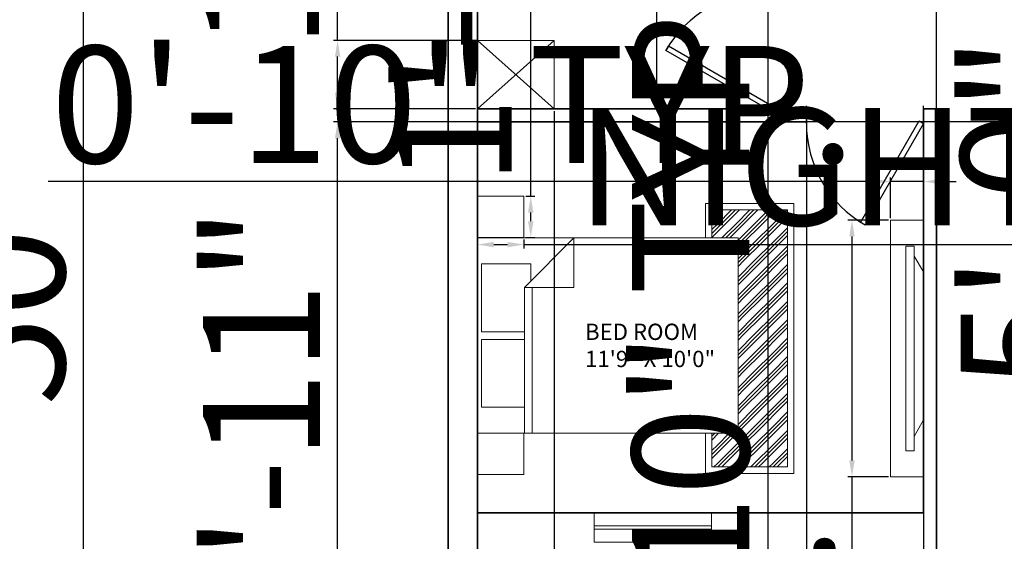
# Model space of a CAD drawing. Units: inches. Extents: x 2901 to 21549, y 2042 to 3828.
# Tile 3 of 10: x 3202 to 3505, y 3099 to 3259. Entities that reach past the tile are written whole.
import ezdxf

# ---------------------------------------------------------------- set-up
doc = ezdxf.new("R2010")
doc.units = ezdxf.units.IN
doc.layers.get('Defpoints').update_dxf_attribs({"color": 1})
for name, color, linetype, lineweight in [('A-ANNO-DIMS', 2, 'Continuous', 18), ('A-AREA-IDEN', 7, 'Continuous', 18), ('A-DOOR', 3, 'Continuous', 25), ('A-EQPM', 8, 'Continuous', 18), ('A-FLOR-FIXT', 9, 'Continuous', 18), ('A-FLOR-PATT', 252, 'Continuous', 13), ('A-FURN', 8, 'Continuous', 18), ('A-GLAZ', 4, 'Continuous', 18), ('A-WALL', 7, 'Continuous', 35)]:
    doc.layers.add(name, color=color, linetype=linetype, lineweight=lineweight)
doc.styles.get("Standard").update_dxf_attribs({"font": 'arial.ttf'})
doc.dimstyles.new('ISO-25', dxfattribs={"dimtxt": 36, "dimasz": 5, "dimexe": 1.25, "dimexo": 0.625, "dimtad": 1, "dimdec": 0, "dimlunit": 3, "dimtxsty": 'Standard', "dimcen": 2.5, "dimadec": 0, "dimazin": 0, "dimtfac": 1, "dimtdec": 0, "dimtmove": 0, "dimatfit": 3, "dimfxl": 1, "dimarcsym": 0})

# ---------------------------------------------------------------- blocks, each defined once
blk = doc.blocks.new('*U22')
for p, q in [((-40, 0), (-40, 6)), ((0, 0), (0, 6))]:
    blk.add_line(p, q)
blk.add_lwpolyline([(0, 0), (-20, -34.64), (-21.52, -33.77), (-1.52, 0.87)], close=True)
blk.add_arc((0, 0), 40, 180, 240)
blk = doc.blocks.new('Bed - Queen')
for p, q in [((0, -80.00003), (0, 0)), ((0, 0), (59.99999, 0)), ((59.99999, 0), (59.99999, -80.00003)), ((7.99999, -1.2), (28.79998, -1.2)), ((7.99999, -14.4), (7.99999, -1.2)), ((28.79998, -1.2), (28.79998, -14.4)), ((31.19999, -1.2), (51.99999, -1.2)), ((31.19999, -14.4), (31.19999, -1.2)), ((51.99999, -1.2), (51.99999, -16.4)), ((0, -14.4), (44.8, -14.4)), ((59.99999, -29.6), (44.8, -14.4)), ((44.8, -14.4), (44.8, -29.6)), ((44.8, -16.8), (0, -16.8)), ((51.99999, -16.4), (46.79936, -16.4)), ((44.8, -29.6), (59.99999, -29.6)), ((59.99999, -80.00003), (0, -80.00003))]:
    blk.add_line(p, q)
blk = doc.blocks.new('*D31')
at = {"layer": 'A-ANNO-DIMS', "color": 0, "lineweight": -2, "transparency": 16777216}
for p, q in [((3333.44, 3474.48), (3220.78, 3474.48)), ((3222.03, 3469.48), (3222.03, 2879.48)), ((3333.44, 2874.48), (3220.78, 2874.48))]:
    blk.add_line(p, q, dxfattribs=at)
at = {"layer": 'A-ANNO-DIMS', "color": 0, "transparency": 16777216}
for points in [[(3221.19, 3469.48), (3222.86, 3469.48), (3222.03, 3474.48)], [(3221.19, 2879.48), (3222.86, 2879.48), (3222.03, 2874.48)]]:
    blk.add_solid(points, dxfattribs=at)
at = {"layer": 'Defpoints', "color": 0, "transparency": 16777216}
for p in [(3334.07, 3474.48), (3222.03, 2874.48), (3334.07, 2874.48)]:
    blk.add_point(p, dxfattribs=at)
at = {"layer": 'A-ANNO-DIMS', "color": 0, "transparency": 16777216, "insert": (3203.02, 3174.48), "char_height": 36, "attachment_point": 5, "rotation": 90}
blk.add_mtext("50'", dxfattribs=at)
blk = doc.blocks.new('WIN-36IN-9IN-WALL')
for p, q in [((0, 36), (9, 36)), ((0, 0), (0, 36)), ((4, 0), (4, 36)), ((5, 36), (5, 0)), ((9, 36), (9, 0)), ((9, 0), (0, 0))]:
    blk.add_line(p, q)
blk = doc.blocks.new('TABLE-BEDSIDE')
blk.add_lwpolyline([(0, 12.7), (14.22, 12.7), (14.22, 0), (0, 0)], close=True)
blk = doc.blocks.new('BEDROOM-MEDIA-UNIT')
for p, q in [((2.89, 66.49), (0, 61.37)), ((0, 15.88), (2.89, 11.11))]:
    blk.add_line(p, q)
for points in [[(0.06, 78.84), (10.18, 78.84), (10.18, 0), (0.06, 0)], [(2.89, 70.84), (5.46, 70.84), (5.46, 8), (2.89, 8)]]:
    blk.add_lwpolyline(points, close=True)
blk = doc.blocks.new('*D38')
at = {"layer": 'A-ANNO-DIMS', "color": 0, "lineweight": -2, "transparency": 16777216}
for p, q in [((3343.07, 3191.34), (3343.07, 3188.58)), ((3348.07, 3189.83), (3352.29, 3189.83)), ((3357.29, 3191.34), (3357.29, 3188.58)), ((3357.29, 3189.83), (3922.11, 3189.83))]:
    blk.add_line(p, q, dxfattribs=at)
at = {"layer": 'A-ANNO-DIMS', "color": 0, "transparency": 16777216}
for points in [[(3348.07, 3190.67), (3348.07, 3189), (3343.07, 3189.83)], [(3352.29, 3190.67), (3352.29, 3189), (3357.29, 3189.83)]]:
    blk.add_solid(points, dxfattribs=at)
at = {"layer": 'Defpoints', "color": 0, "transparency": 16777216}
for p in [(3343.07, 3191.97), (3357.29, 3191.97), (3357.29, 3189.83)]:
    blk.add_point(p, dxfattribs=at)
at = {"layer": 'A-ANNO-DIMS', "color": 0, "transparency": 16777216, "insert": (3642.2, 3209.07), "char_height": 36, "attachment_point": 5}
blk.add_mtext('NIGHTSTAND 1\'-2" TYP.', dxfattribs=at)
blk = doc.blocks.new('*D39')
at = {"layer": 'A-ANNO-DIMS', "color": 0, "lineweight": -2, "transparency": 16777216}
for p, q in [((3359.43, 3204.67), (3359.43, 3510.85)), ((3357.92, 3204.67), (3360.68, 3204.67)), ((3359.43, 3196.97), (3359.43, 3199.67)), ((3357.92, 3191.97), (3360.68, 3191.97))]:
    blk.add_line(p, q, dxfattribs=at)
at = {"layer": 'A-ANNO-DIMS', "color": 0, "transparency": 16777216}
for points in [[(3358.59, 3199.67), (3360.26, 3199.67), (3359.43, 3204.67)], [(3358.59, 3196.97), (3360.26, 3196.97), (3359.43, 3191.97)]]:
    blk.add_solid(points, dxfattribs=at)
at = {"layer": 'Defpoints', "color": 0, "transparency": 16777216}
for p in [(3357.29, 3204.67), (3359.43, 3204.67), (3357.29, 3191.97)]:
    blk.add_point(p, dxfattribs=at)
at = {"layer": 'A-ANNO-DIMS', "color": 0, "transparency": 16777216, "insert": (3340.19, 3360.26), "char_height": 36, "attachment_point": 5, "rotation": 90}
blk.add_mtext('1\'-0 1/2" TYP.', dxfattribs=at)
blk = doc.blocks.new('*D40')
at = {"layer": 'A-ANNO-DIMS', "color": 0, "lineweight": -2, "transparency": 16777216}
for p, q in [((3343.07, 3272.69), (3343.07, 3267.11)), ((3376.12, 3272.69), (3376.12, 3267.11)), ((3343.07, 3268.36), (3018.15, 3268.36)), ((3371.12, 3268.36), (3348.07, 3268.36))]:
    blk.add_line(p, q, dxfattribs=at)
at = {"layer": 'A-ANNO-DIMS', "color": 0, "transparency": 16777216}
for points in [[(3348.07, 3269.19), (3348.07, 3267.52), (3343.07, 3268.36)], [(3371.12, 3269.19), (3371.12, 3267.52), (3376.12, 3268.36)]]:
    blk.add_solid(points, dxfattribs=at)
at = {"layer": 'Defpoints', "color": 0, "transparency": 16777216}
for p in [(3343.07, 3273.32), (3376.12, 3273.32), (3343.07, 3268.36)]:
    blk.add_point(p, dxfattribs=at)
at = {"layer": 'A-ANNO-DIMS', "color": 0, "transparency": 16777216, "insert": (3178.11, 3287.6), "char_height": 36, "attachment_point": 5}
blk.add_mtext('WC 2\'-9" TYP.', dxfattribs=at)
blk = doc.blocks.new('*D42')
at = {"layer": 'A-ANNO-DIMS', "color": 0, "lineweight": -2, "transparency": 16777216}
for p, q in [((3533.42, 3266.44), (3528.38, 3599.53)), ((3535.49, 3266.47), (3532.17, 3266.42)), ((3533.62, 3253.49), (3533.5, 3261.44)), ((3535.76, 3248.52), (3532.44, 3248.47))]:
    blk.add_line(p, q, dxfattribs=at)
at = {"layer": 'A-ANNO-DIMS', "color": 0, "transparency": 16777216}
for points in [[(3534.33, 3261.45), (3532.66, 3261.43), (3533.42, 3266.44)], [(3534.45, 3253.5), (3532.78, 3253.48), (3533.69, 3248.49)]]:
    blk.add_solid(points, dxfattribs=at)
at = {"layer": 'Defpoints', "color": 0, "transparency": 16777216}
for p in [(3533.42, 3266.44), (3536.11, 3266.48), (3536.39, 3248.53)]:
    blk.add_point(p, dxfattribs=at)
at = {"layer": 'A-ANNO-DIMS', "color": 0, "transparency": 16777216, "insert": (3549.86, 3435.77), "char_height": 36, "attachment_point": 5, "rotation": 270.8679}
blk.add_mtext('LAV 1\'-6" TYP.', dxfattribs=at)
blk = doc.blocks.new('*D44')
at = {"layer": 'A-ANNO-DIMS', "color": 0, "lineweight": -2, "transparency": 16777216}
for p, q in [((3432.19, 3305.97), (3432.19, 3310.97)), ((3431.32, 3300.97), (3433.44, 3300.97)), ((3432.19, 3300.97), (3432.19, 3290.97)), ((3431.32, 3290.97), (3433.44, 3290.97)), ((3432.19, 3285.97), (3432.19, 2919.63))]:
    blk.add_line(p, q, dxfattribs=at)
at = {"layer": 'A-ANNO-DIMS', "color": 0, "transparency": 16777216}
for points in [[(3431.36, 3305.97), (3433.02, 3305.97), (3432.19, 3300.97)], [(3431.36, 3285.97), (3433.02, 3285.97), (3432.19, 3290.97)]]:
    blk.add_solid(points, dxfattribs=at)
at = {"layer": 'Defpoints', "color": 0, "transparency": 16777216}
for p in [(3430.69, 3300.97), (3430.69, 3290.97), (3432.19, 3290.97)]:
    blk.add_point(p, dxfattribs=at)
at = {"layer": 'A-ANNO-DIMS', "color": 0, "transparency": 16777216, "insert": (3413.18, 3100.3), "char_height": 36, "attachment_point": 5, "rotation": 90}
blk.add_mtext('TAP 0\'-10" TYP.', dxfattribs=at)
blk = doc.blocks.new('*D45')
at = {"layer": 'A-ANNO-DIMS', "color": 0, "lineweight": -2, "transparency": 16777216}
for p, q in [((3419.19, 3302.47), (3414.19, 3302.47)), ((3424.19, 3301.6), (3424.19, 3303.72)), ((3424.19, 3302.47), (3430.69, 3302.47)), ((3430.69, 3301.6), (3430.69, 3303.72)), ((3435.69, 3302.47), (3745.26, 3302.47))]:
    blk.add_line(p, q, dxfattribs=at)
at = {"layer": 'A-ANNO-DIMS', "color": 0, "transparency": 16777216}
for points in [[(3419.19, 3303.31), (3419.19, 3301.64), (3424.19, 3302.47)], [(3435.69, 3303.31), (3435.69, 3301.64), (3430.69, 3302.47)]]:
    blk.add_solid(points, dxfattribs=at)
at = {"layer": 'Defpoints', "color": 0, "transparency": 16777216}
for p in [(3430.69, 3302.47), (3424.19, 3300.97), (3430.69, 3300.97)]:
    blk.add_point(p, dxfattribs=at)
at = {"layer": 'A-ANNO-DIMS', "color": 0, "transparency": 16777216, "insert": (3592.98, 3321.71), "char_height": 36, "attachment_point": 5}
blk.add_mtext('0\'-6 1/2" TYP.', dxfattribs=at)
blk = doc.blocks.new('*D47')
at = {"layer": 'A-ANNO-DIMS', "color": 0, "lineweight": -2, "transparency": 16777216}
for p, q in [((3544.44, 3430.67), (3531.82, 3430.67)), ((3533.07, 3425.67), (3533.07, 3375.67)), ((3544.44, 3370.67), (3531.82, 3370.67)), ((3533.07, 3370.67), (3533.07, 3144.99))]:
    blk.add_line(p, q, dxfattribs=at)
at = {"layer": 'A-ANNO-DIMS', "color": 0, "transparency": 16777216}
for points in [[(3532.24, 3425.67), (3533.9, 3425.67), (3533.07, 3430.67)], [(3532.24, 3375.67), (3533.9, 3375.67), (3533.07, 3370.67)]]:
    blk.add_solid(points, dxfattribs=at)
at = {"layer": 'Defpoints', "color": 0, "transparency": 16777216}
for p in [(3545.07, 3430.67), (3533.07, 3370.67), (3545.07, 3370.67)]:
    blk.add_point(p, dxfattribs=at)
at = {"layer": 'A-ANNO-DIMS', "color": 0, "transparency": 16777216, "insert": (3514.06, 3255.33), "char_height": 36, "attachment_point": 5, "rotation": 90}
blk.add_mtext('5\'-0" TYP.', dxfattribs=at)
blk = doc.blocks.new('*D52')
at = {"layer": 'A-ANNO-DIMS', "color": 0, "lineweight": -2, "transparency": 16777216}
for p, q in [((3469.26, 3197.35), (3456.81, 3197.35)), ((3458.06, 3192.35), (3458.06, 3123.52)), ((3469.26, 3118.52), (3456.81, 3118.52)), ((3458.06, 3118.52), (3458.06, 2589.92))]:
    blk.add_line(p, q, dxfattribs=at)
at = {"layer": 'A-ANNO-DIMS', "color": 0, "transparency": 16777216}
for points in [[(3457.23, 3192.35), (3458.9, 3192.35), (3458.06, 3197.35)], [(3457.23, 3123.52), (3458.9, 3123.52), (3458.06, 3118.52)]]:
    blk.add_solid(points, dxfattribs=at)
at = {"layer": 'Defpoints', "color": 0, "transparency": 16777216}
for p in [(3469.89, 3197.35), (3458.06, 3118.52), (3469.89, 3118.52)]:
    blk.add_point(p, dxfattribs=at)
at = {"layer": 'A-ANNO-DIMS', "color": 0, "transparency": 16777216, "insert": (3439.06, 2851.72), "char_height": 36, "attachment_point": 5, "rotation": 90}
blk.add_mtext('MEDIA UNIT 6\'-7" TYP.', dxfattribs=at)
blk = doc.blocks.new('*D53')
at = {"layer": 'A-ANNO-DIMS', "color": 0, "lineweight": -2, "transparency": 16777216}
for p, q in [((3464.89, 3209.18), (3211.23, 3209.18)), ((3469.89, 3197.98), (3469.89, 3210.43)), ((3480.07, 3209.18), (3469.89, 3209.18)), ((3480.07, 3197.98), (3480.07, 3210.43)), ((3485.07, 3209.18), (3490.07, 3209.18))]:
    blk.add_line(p, q, dxfattribs=at)
at = {"layer": 'A-ANNO-DIMS', "color": 0, "transparency": 16777216}
for points in [[(3464.89, 3210.01), (3464.89, 3208.34), (3469.89, 3209.18)], [(3485.07, 3210.01), (3485.07, 3208.34), (3480.07, 3209.18)]]:
    blk.add_solid(points, dxfattribs=at)
at = {"layer": 'Defpoints', "color": 0, "transparency": 16777216}
for p in [(3469.89, 3209.18), (3469.89, 3197.35), (3480.07, 3197.35)]:
    blk.add_point(p, dxfattribs=at)
at = {"layer": 'A-ANNO-DIMS', "color": 0, "transparency": 16777216, "insert": (3335.56, 3228.18), "char_height": 36, "attachment_point": 5}
blk.add_mtext('0\'-10" TYP.', dxfattribs=at)
blk = doc.blocks.new('*D67')
at = {"layer": 'A-ANNO-DIMS', "color": 0, "lineweight": -2, "transparency": 16777216}
for p, q in [((3484.07, 3013.1), (3484.07, 3509.68)), ((3489.07, 3508.43), (3620.07, 3508.43)), ((3625.07, 3228.1), (3625.07, 3509.68))]:
    blk.add_line(p, q, dxfattribs=at)
at = {"layer": 'A-ANNO-DIMS', "color": 0, "transparency": 16777216}
for points in [[(3489.07, 3509.26), (3489.07, 3507.59), (3484.07, 3508.43)], [(3620.07, 3509.26), (3620.07, 3507.59), (3625.07, 3508.43)]]:
    blk.add_solid(points, dxfattribs=at)
at = {"layer": 'Defpoints', "color": 0, "transparency": 16777216}
for p in [(3625.07, 3508.43), (3625.07, 3227.48), (3484.07, 3012.48)]:
    blk.add_point(p, dxfattribs=at)
at = {"layer": 'A-ANNO-DIMS', "color": 0, "transparency": 16777216, "insert": (3554.57, 3527.43), "char_height": 36, "attachment_point": 5}
blk.add_mtext('11\'-9"', dxfattribs=at)
blk = doc.blocks.new('*D68')
at = {"layer": 'A-ANNO-DIMS', "color": 0, "lineweight": -2, "transparency": 16777216}
for p, q in [((3531.44, 3227.48), (3298.87, 3227.48)), ((3300.12, 3017.48), (3300.12, 3222.48)), ((3483.44, 3012.48), (3298.87, 3012.48))]:
    blk.add_line(p, q, dxfattribs=at)
at = {"layer": 'A-ANNO-DIMS', "color": 0, "transparency": 16777216}
for points in [[(3299.29, 3222.48), (3300.95, 3222.48), (3300.12, 3227.48)], [(3299.29, 3017.48), (3300.95, 3017.48), (3300.12, 3012.48)]]:
    blk.add_solid(points, dxfattribs=at)
at = {"layer": 'Defpoints', "color": 0, "transparency": 16777216}
for p in [(3300.12, 3227.48), (3532.07, 3227.48), (3484.07, 3012.48)]:
    blk.add_point(p, dxfattribs=at)
at = {"layer": 'A-ANNO-DIMS', "color": 0, "transparency": 16777216, "insert": (3281.42, 3119.98), "char_height": 36, "attachment_point": 5, "rotation": 90}
blk.add_mtext('17\'-11"', dxfattribs=at)
blk = doc.blocks.new('*D78')
at = {"layer": 'A-ANNO-DIMS', "color": 0, "lineweight": -2, "transparency": 16777216}
for p, q in [((3343.07, 3230.85), (3343.07, 2839.28)), ((3366.66, 3230.85), (3366.66, 2839.28)), ((3348.07, 2840.53), (3361.66, 2840.53)), ((3366.66, 2840.53), (3577.07, 2840.53))]:
    blk.add_line(p, q, dxfattribs=at)
at = {"layer": 'A-ANNO-DIMS', "color": 0, "transparency": 16777216}
for points in [[(3348.07, 2841.36), (3348.07, 2839.69), (3343.07, 2840.53)], [(3361.66, 2841.36), (3361.66, 2839.69), (3366.66, 2840.53)]]:
    blk.add_solid(points, dxfattribs=at)
at = {"layer": 'Defpoints', "color": 0, "transparency": 16777216}
for p in [(3343.07, 3231.48), (3366.66, 3231.48), (3366.66, 2840.53)]:
    blk.add_point(p, dxfattribs=at)
at = {"layer": 'A-ANNO-DIMS', "color": 0, "transparency": 16777216, "insert": (3474.37, 2859.77), "char_height": 36, "attachment_point": 5}
blk.add_mtext('1\'-11 1/2"', dxfattribs=at)
blk = doc.blocks.new('*D79')
at = {"layer": 'A-ANNO-DIMS', "color": 0, "lineweight": -2, "transparency": 16777216}
for p, q in [((3300.12, 3252.55), (3300.12, 3351.11)), ((3342.44, 3252.55), (3298.87, 3252.55)), ((3300.12, 3236.48), (3300.12, 3247.55)), ((3342.44, 3231.48), (3298.87, 3231.48))]:
    blk.add_line(p, q, dxfattribs=at)
at = {"layer": 'A-ANNO-DIMS', "color": 0, "transparency": 16777216}
for points in [[(3299.29, 3247.55), (3300.95, 3247.55), (3300.12, 3252.55)], [(3299.29, 3236.48), (3300.95, 3236.48), (3300.12, 3231.48)]]:
    blk.add_solid(points, dxfattribs=at)
at = {"layer": 'Defpoints', "color": 0, "transparency": 16777216}
for p in [(3300.12, 3252.55), (3343.07, 3252.55), (3343.07, 3231.48)]:
    blk.add_point(p, dxfattribs=at)
at = {"layer": 'A-ANNO-DIMS', "color": 0, "transparency": 16777216, "insert": (3281.11, 3304.33), "char_height": 36, "attachment_point": 5, "rotation": 90}
blk.add_mtext('1\'-9"', dxfattribs=at)
blk = doc.blocks.new('*D83')
at = {"layer": 'A-ANNO-DIMS', "color": 0, "lineweight": -2, "transparency": 16777216}
for p, q in [((3398.12, 3267.48), (3398.12, 3369.4)), ((3431.44, 3267.48), (3396.87, 3267.48)), ((3398.12, 3236.48), (3398.12, 3262.48)), ((3431.44, 3231.48), (3396.87, 3231.48))]:
    blk.add_line(p, q, dxfattribs=at)
at = {"layer": 'A-ANNO-DIMS', "color": 0, "transparency": 16777216}
for points in [[(3397.29, 3262.48), (3398.95, 3262.48), (3398.12, 3267.48)], [(3397.29, 3236.48), (3398.95, 3236.48), (3398.12, 3231.48)]]:
    blk.add_solid(points, dxfattribs=at)
at = {"layer": 'Defpoints', "color": 0, "transparency": 16777216}
for p in [(3398.12, 3267.48), (3432.07, 3267.48), (3432.07, 3231.48)]:
    blk.add_point(p, dxfattribs=at)
at = {"layer": 'A-ANNO-DIMS', "color": 0, "transparency": 16777216, "insert": (3379.1, 3320.94), "char_height": 36, "attachment_point": 5, "rotation": 90}
blk.add_mtext('3\'-0"', dxfattribs=at)
blk = doc.blocks.new('*D84')
at = {"layer": 'A-ANNO-DIMS', "color": 0, "lineweight": -2, "transparency": 16777216}
for p, q in [((3444.07, 3230.85), (3444.07, 2839.28)), ((3480.07, 3230.85), (3480.07, 2839.28)), ((3449.07, 2840.53), (3475.07, 2840.53)), ((3480.07, 2840.53), (3581.99, 2840.53))]:
    blk.add_line(p, q, dxfattribs=at)
at = {"layer": 'A-ANNO-DIMS', "color": 0, "transparency": 16777216}
for points in [[(3449.07, 2841.36), (3449.07, 2839.69), (3444.07, 2840.53)], [(3475.07, 2841.36), (3475.07, 2839.69), (3480.07, 2840.53)]]:
    blk.add_solid(points, dxfattribs=at)
at = {"layer": 'Defpoints', "color": 0, "transparency": 16777216}
for p in [(3444.07, 3231.48), (3480.07, 3231.48), (3480.07, 2840.53)]:
    blk.add_point(p, dxfattribs=at)
at = {"layer": 'A-ANNO-DIMS', "color": 0, "transparency": 16777216, "insert": (3533.53, 2859.55), "char_height": 36, "attachment_point": 5}
blk.add_mtext('3\'-0"', dxfattribs=at)

msp = doc.modelspace()

# ---------------------------------------------------------------- hatches: boundary and pattern name
at = {"layer": 'A-FLOR-PATT'}
h = msp.add_hatch(dxfattribs=at)
h.set_pattern_fill('GOST_GROUND', color=256, scale=0.4)
h.paths.add_polyline_path([(3438.25, 3200.47), (3415.05, 3200.47), (3415.05, 3191.87), (3423.07, 3191.87), (3423.07, 3131.87), (3415.05, 3131.87), (3415.05, 3121.53), (3438.25, 3121.53)])

# ---------------------------------------------------------------- linework, layer by layer
at = {"layer": 'A-EQPM'}
msp.add_line((3480.07, 3135.98), (3480.07, 3181.48), dxfattribs=at)
at = {"layer": 'A-FLOR-FIXT'}
for p, q in [((3343.07, 3231.48), (3366.66, 3252.55)), ((3366.66, 3231.48), (3343.07, 3252.55))]:
    msp.add_line(p, q, dxfattribs=at)
msp.add_lwpolyline([(3343.07, 3252.55), (3366.66, 3252.55), (3366.66, 3231.48), (3343.07, 3231.48)], close=True, dxfattribs=at)
at = {"layer": 'A-FURN'}
for points in [[(3413.05, 3191.87), (3413.05, 3202.47), (3440.25, 3202.47), (3440.25, 3119.53)], [(3415.05, 3191.87), (3415.05, 3200.47), (3438.25, 3200.47), (3438.25, 3121.53), (3415.05, 3121.53), (3415.05, 3131.87)], [(3440.25, 3130.12), (3440.25, 3119.53), (3413.05, 3119.53), (3413.05, 3131.87)]]:
    msp.add_lwpolyline(points, dxfattribs=at)
at = {"layer": 'A-WALL'}
for p, q in [((3343.07, 2883.48), (3343.07, 3465.48)), ((3343.07, 3231.48), (3444.07, 3231.48)), ((3432.07, 3231.48), (3436.07, 3231.48)), ((3436.07, 3231.48), (3436.07, 3227.48)), ((3444.07, 3227.48), (3444.07, 3231.48)), ((3480.07, 3107.48), (3480.07, 3231.48)), ((3480.07, 3231.48), (3484.07, 3231.48)), ((3484.07, 3012.48), (3484.07, 3231.48)), ((3343.07, 3227.48), (3444.07, 3227.48)), ((3436.07, 3227.48), (3436.07, 3227.48)), ((3343.07, 3107.48), (3480.07, 3107.48))]:
    msp.add_line(p, q, dxfattribs=at)
msp.add_lwpolyline([(3634.07, 3474.48), (3634.07, 2874.48), (3334.07, 2874.48), (3334.07, 3474.48)], close=True, dxfattribs=at)

# ---------------------------------------------------------------- block references
at = {"layer": 'A-DOOR', "xscale": 0.8999999999999889, "yscale": 0.8999999999999889, "zscale": 0.8999999999999889, "rotation": 270.0000000000072}
msp.add_blockref('*U22', (3432.07, 3231.48), dxfattribs=at)
at = {"layer": 'A-DOOR', "xscale": 0.9, "yscale": 0.9, "zscale": 0.9}
msp.add_blockref('*U22', (3480.07, 3227.03), dxfattribs=at)
at = {"layer": 'A-EQPM', "rotation": 180}
msp.add_blockref('BEDROOM-MEDIA-UNIT', (3480.07, 3197.35), dxfattribs=at)
at = {"layer": 'A-FURN'}
for p in [(3343.07, 3191.97), (3343.07, 3119.17)]:
    msp.add_blockref('TABLE-BEDSIDE', p, dxfattribs=at)
at = {"layer": 'A-FURN', "rotation": 90}
msp.add_blockref('Bed - Queen', (3343.07, 3131.87), dxfattribs=at)
at = {"layer": 'A-GLAZ', "rotation": 270}
msp.add_blockref('WIN-36IN-9IN-WALL', (3378.91, 3107.48), dxfattribs=at)

# ---------------------------------------------------------------- texts
at = {"layer": 'A-AREA-IDEN', "insert": (3376.09, 3165.54), "char_height": 5, "attachment_point": 1}
msp.add_mtext_dynamic_manual_height_columns('{\\fArial|b1|i0|c0|p34;BED ROOM\\P11\'9" X 10\'0"}', width=86.7973, gutter_width=12.5, heights=[27.4], dxfattribs=at)

# ---------------------------------------------------------------- dimensions: what is measured, and where the dimension line sits
at = {"layer": 'A-ANNO-DIMS'}
for base, p1, p2, angle, text, picture, middle in [((3533.42, 3266.44), (3536.39, 3248.53), (3536.11, 3266.48), 90.8679, 'LAV <> TYP.', '*D42', (3549.86, 3435.77)), ((3359.43, 3204.67), (3357.29, 3191.97), (3357.29, 3204.67), 90, '<> TYP.', '*D39', (3340.19, 3360.26)), ((3533.07, 3370.67), (3545.07, 3430.67), (3545.07, 3370.67), 270, '<> TYP.', '*D47', (3514.06, 3255.33)), ((3343.0696, 3268.3583), (3376.1159, 3273.3152), (3343.0696, 3273.3152), 180, 'WC <> TYP.', '*D40', (3178.109, 3287.5972)), ((3432.19, 3290.97), (3430.69, 3300.97), (3430.69, 3290.97), 270, 'TAP <> TYP.', '*D44', (3413.18, 3100.3)), ((3469.89, 3209.18), (3480.07, 3197.35), (3469.89, 3197.35), 180, '<> TYP.', '*D53', (3335.56, 3228.18)), ((3458.06, 3118.52), (3469.89, 3197.35), (3469.89, 3118.52), 270, 'MEDIA UNIT <> TYP.', '*D52', (3439.06, 2851.72))]:
    dim = msp.add_linear_dim(base=base, p1=p1, p2=p2, angle=angle, text=text, dimstyle='ISO-25', override={"dimdec": 1, "dimlfac": 1, "dimrnd": 0, "dimzin": 1, "dimdsep": 46, "dimlunit": 4, "dimfrac": 2}, dxfattribs=at)
    dim.commit()
    dim.dimension.update_dxf_attribs({"geometry": picture, "text_midpoint": middle})
for base, p1, p2, picture, middle in [((3625.07, 3508.43), (3484.07, 3012.48), (3625.07, 3227.48), '*D67', (3554.57, 3527.43)), ((3366.66, 2840.53), (3343.07, 3231.48), (3366.66, 3231.48), '*D78', (3474.37, 2859.77)), ((3480.07, 2840.53), (3444.07, 3231.48), (3480.07, 3231.48), '*D84', (3533.53, 2859.55))]:
    dim = msp.add_linear_dim(base=base, p1=p1, p2=p2, dimstyle='ISO-25', override={"dimdec": 1, "dimlfac": 1, "dimrnd": 0, "dimzin": 1, "dimdsep": 46, "dimlunit": 4, "dimfrac": 2}, dxfattribs=at)
    dim.commit()
    dim.dimension.update_dxf_attribs({"geometry": picture, "text_midpoint": middle})
for base, p1, p2, override, picture, middle in [((3222.03, 2874.48), (3334.07, 3474.48), (3334.07, 2874.48), {"dimclrd": 0, "dimclre": 0, "dimclrt": 0}, '*D31', (3203.02, 3174.48)), ((3398.12, 3267.48), (3432.07, 3231.48), (3432.07, 3267.48), {"dimdec": 1, "dimlfac": 1, "dimrnd": 0, "dimzin": 1, "dimdsep": 46, "dimlunit": 4, "dimfrac": 2}, '*D83', (3379.1, 3320.94)), ((3300.12, 3252.55), (3343.07, 3231.48), (3343.07, 3252.55), {"dimdec": 1, "dimlfac": 1, "dimrnd": 0, "dimzin": 1, "dimdsep": 46, "dimlunit": 4, "dimfrac": 2}, '*D79', (3281.11, 3304.33)), ((3300.12, 3227.48), (3484.07, 3012.48), (3532.07, 3227.48), {"dimdec": 1, "dimlfac": 1, "dimrnd": 0, "dimzin": 1, "dimdsep": 46, "dimlunit": 4, "dimfrac": 2}, '*D68', (3281.42, 3119.98))]:
    dim = msp.add_linear_dim(base=base, p1=p1, p2=p2, angle=90, dimstyle='ISO-25', override=override, dxfattribs=at)
    dim.commit()
    dim.dimension.update_dxf_attribs({"geometry": picture, "text_midpoint": middle})
for base, p1, p2, text, picture, middle in [((3430.69, 3302.47), (3424.19, 3300.97), (3430.69, 3300.97), '<> TYP.', '*D45', (3592.98, 3321.71)), ((3357.29, 3189.83), (3343.07, 3191.97), (3357.29, 3191.97), 'NIGHTSTAND <> TYP.', '*D38', (3642.2, 3209.07))]:
    dim = msp.add_linear_dim(base=base, p1=p1, p2=p2, text=text, dimstyle='ISO-25', override={"dimdec": 1, "dimlfac": 1, "dimrnd": 0, "dimzin": 1, "dimdsep": 46, "dimlunit": 4, "dimfrac": 2}, dxfattribs=at)
    dim.commit()
    dim.dimension.update_dxf_attribs({"geometry": picture, "text_midpoint": middle})

doc.saveas('drawing.dxf')
